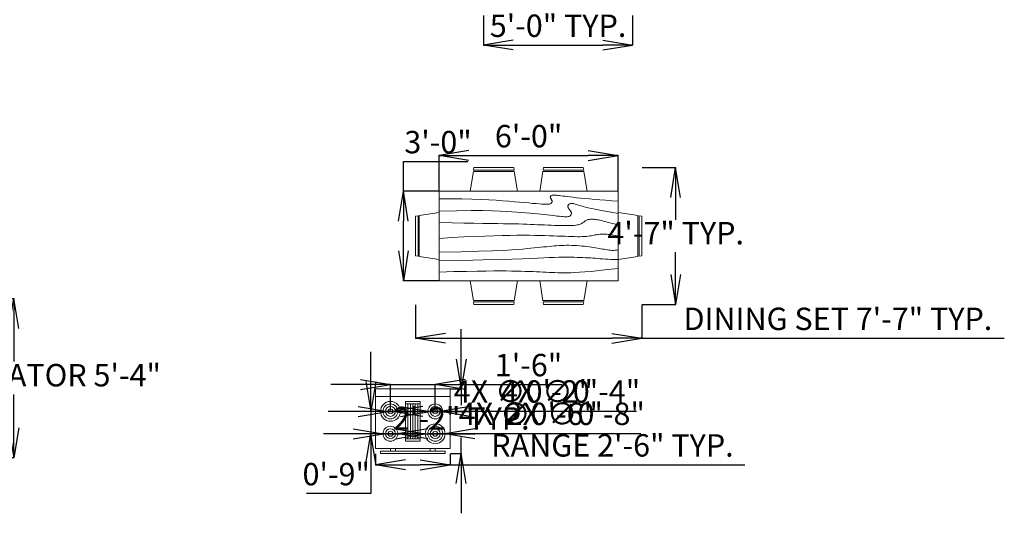
# Model space of a CAD drawing. Units: inches. Extents: x 1856 to 3350, y 1624 to 2224.
# Tile 6 of 7: x 2954 to 3350, y 1624 to 1823. Entities that reach past the tile are written whole.
import ezdxf

# ---------------------------------------------------------------- set-up
doc = ezdxf.new("R2010")
doc.units = ezdxf.units.IN
for name, color, linetype, lineweight in [('A-ANNO-DIMS', 2, 'Continuous', 18), ('A-EQPM', 3, 'Continuous', 18), ('A-FURN', 3, 'Continuous', 18)]:
    doc.layers.add(name, color=color, linetype=linetype, lineweight=lineweight)
doc.styles.get("Standard").update_dxf_attribs({"font": 'arial.ttf'})
doc.dimstyles.new('ISO-25', dxfattribs={"dimtxt": 9, "dimasz": 12, "dimexe": 0.125, "dimexo": 0.125, "dimgap": 2, "dimtad": 1, "dimtih": 1, "dimtoh": 1, "dimdec": 1, "dimzin": 11, "dimlunit": 4, "dimtxsty": 'Standard', "dimblk": 'OPEN', "dimcen": -0.125, "dimadec": 0, "dimazin": 0, "dimtfac": 1, "dimtdec": 1, "dimtmove": 0, "dimatfit": 3, "dimfxl": 1, "dimarcsym": 0})

# ---------------------------------------------------------------- blocks, each defined once
blk = doc.blocks.new('Dining Set - 36 x 72 in.')
for p, q in [((-22.2343, 26.00059), (-23.4847, 17.99762)), ((-22.2304, 26), (-5.7608, 26)), ((-22, 27.5), (-22.1562, 26.50042)), ((-5.8416, 26.5), (-22.1534, 26.5)), ((-22, 27.5), (-6, 27.5)), ((-5.8437, 26.49966), (-6, 27.5)), ((-4.5152, 17.99762), (-5.7655, 25.99926)), ((5.7657, 26.00059), (4.5153, 17.99762)), ((5.7696, 26), (22.2392, 26)), ((6, 27.5), (5.8438, 26.50042)), ((22.1584, 26.5), (5.8466, 26.5)), ((6, 27.5), (22, 27.5)), ((22.1563, 26.49966), (22, 27.5)), ((23.4848, 17.99762), (22.2345, 25.99926)), ((36, 18), (-36, 18)), ((-36, 18), (-36, -18)), ((36, -18), (36, 18)), ((-45.5, 8), (-44.5004, 8.15617)), ((-45.5, 8), (-45.5, -8)), ((-44.5, -8.15843), (-44.5, 8.15338)), ((-44.0006, 8.23428), (-35.9976, 9.48474)), ((-44, 8.23041), (-44, -8.23915)), ((44.0006, 8.23428), (35.9976, 9.48474)), ((44, 8.23041), (44, -8.23915)), ((44.5, -8.15843), (44.5, 8.15338)), ((45.5, 8), (44.5005, 8.15617)), ((45.5, 8), (45.5, -8)), ((-44.4997, -8.15631), (-45.5, -8)), ((-35.9976, -9.48476), (-43.9993, -8.2345)), ((35.9976, -9.48476), (43.9993, -8.2345)), ((44.4997, -8.15631), (45.5, -8)), ((-36, -18), (36, -18)), ((-22.2343, -26.0006), (-23.4847, -17.99762)), ((-4.5152, -17.99762), (-5.7655, -25.99928)), ((5.7657, -26.0006), (4.5153, -17.99762)), ((23.4848, -17.99762), (22.2345, -25.99928)), ((-22.2304, -26), (-5.7608, -26)), ((-22, -27.5), (-22.1562, -26.50044)), ((-5.8416, -26.5), (-22.1534, -26.5)), ((-22, -27.5), (-6, -27.5)), ((-5.8437, -26.49967), (-6, -27.5)), ((5.7696, -26), (22.2392, -26)), ((6, -27.5), (5.8438, -26.50044)), ((22.1584, -26.5), (5.8466, -26.5)), ((6, -27.5), (22, -27.5)), ((22.1563, -26.49967), (22, -27.5))]:
    blk.add_line(p, q)
for points in [[(-36, 15), (-31.1772, 14.97754), (-26.8079, 14.91406), (-22.8538, 14.81543), (-19.276, 14.6875), (-16.0362, 14.53613), (-13.0957, 14.36718), (-10.4159, 14.18652), (-7.9583, 14), (-5.6904, 13.81315), (-3.6035, 13.63021), (-1.6954, 13.45508), (0.0365, 13.29166), (1.5945, 13.14388), (2.9811, 13.01562), (4.1988, 12.9108), (5.25, 12.83333), (6.1393, 12.78613), (6.8802, 12.76823), (7.4883, 12.77767), (7.9792, 12.8125), (8.3685, 12.87077), (8.6719, 12.95052), (8.9049, 13.0498), (9.0833, 13.16666), (9.2205, 13.29899), (9.3216, 13.44401), (9.3895, 13.59879), (9.4271, 13.76041), (9.4373, 13.92594), (9.4232, 14.09245), (9.3875, 14.257), (9.3333, 14.41666), (9.2638, 14.56917), (9.1836, 14.71484), (9.0975, 14.85465), (9.0104, 14.98958), (8.9272, 15.1206), (8.8529, 15.2487), (8.7922, 15.37483), (8.75, 15.5), (8.7305, 15.62467), (8.7344, 15.74739), (8.7617, 15.86621), (8.8125, 15.97916), (8.8867, 16.08431), (8.9844, 16.17968), (9.1055, 16.26334), (9.25, 16.33333), (9.4189, 16.38802), (9.6172, 16.42708), (9.8506, 16.45052), (10.125, 16.45833), (10.4463, 16.45052), (10.8203, 16.42708), (11.2529, 16.38802), (11.75, 16.33333), (12.3184, 16.26318), (12.9694, 16.17838), (13.7151, 16.07991), (14.5677, 15.96875), (15.5395, 15.84586), (16.6426, 15.71224), (17.8893, 15.56884), (19.2917, 15.41666), (20.859, 15.25667), (22.5879, 15.08984), (24.4721, 14.91715), (26.5052, 14.73958), (28.6809, 14.5581), (30.9929, 14.3737), (33.4347, 14.18733), (36, 14)], [(-36, 10), (-28.9766, 10.14274), (-23.1725, 10.20442), (-18.4241, 10.19775), (-14.5677, 10.13541), (-11.4399, 10.03011), (-8.877, 9.89453), (-6.7154, 9.74137), (-4.7917, 9.58333), (-2.9698, 9.43082), (-1.2246, 9.28515), (0.4415, 9.14534), (2.026, 9.01041), (3.5266, 8.87939), (4.9408, 8.7513), (6.266, 8.62516), (7.5, 8.5), (8.6411, 8.37549), (9.6914, 8.2539), (10.6538, 8.13818), (11.5312, 8.03125), (12.3267, 7.93603), (13.043, 7.85547), (13.6831, 7.79248), (14.25, 7.75), (14.7471, 7.7303), (15.1797, 7.73307), (15.5537, 7.75732), (15.875, 7.80208), (16.1494, 7.86637), (16.3828, 7.94922), (16.5811, 8.04964), (16.75, 8.16666), (16.8944, 8.29915), (17.0143, 8.44531), (17.1089, 8.60319), (17.1771, 8.77083), (17.218, 8.94629), (17.2305, 9.1276), (17.2137, 9.31282), (17.1667, 9.5), (17.0895, 9.6875), (16.987, 9.875), (16.8649, 10.0625), (16.7292, 10.25), (16.5856, 10.4375), (16.4401, 10.625), (16.2985, 10.8125), (16.1667, 11), (16.05, 11.18733), (15.9518, 11.3737), (15.8752, 11.5581), (15.8229, 11.73958), (15.798, 11.91715), (15.8034, 12.08984), (15.842, 12.25667), (15.9167, 12.41666), (16.0295, 12.56836), (16.1784, 12.70833), (16.3605, 12.83268), (16.5729, 12.9375), (16.8127, 13.01888), (17.0768, 13.07291), (17.3625, 13.0957), (17.6667, 13.08333), (17.9894, 13.03312), (18.3418, 12.94726), (18.7382, 12.82918), (19.1927, 12.68229), (19.7195, 12.51001), (20.3327, 12.31575), (21.0465, 12.10294), (21.875, 11.875), (22.8357, 11.63354), (23.959, 11.37304), (25.2786, 11.08618), (26.8282, 10.76562), (28.6414, 10.40405), (30.752, 9.99414), (33.1936, 9.52856), (36, 9)], [(-36, 5.5), (-30.7157, 5.3348), (-26.069, 5.20963), (-21.9946, 5.11767), (-18.4271, 5.05208), (-15.3009, 5.00602), (-12.5508, 4.97265), (-10.1112, 4.94515), (-7.9167, 4.91666), (-5.909, 4.88167), (-4.0586, 4.83984), (-2.3429, 4.79215), (-0.7396, 4.73958), (0.7739, 4.6831), (2.22, 4.6237), (3.6213, 4.56233), (5, 4.5), (6.373, 4.43782), (7.7344, 4.3776), (9.0723, 4.32129), (10.375, 4.27083), (11.6309, 4.22819), (12.8281, 4.19531), (13.9551, 4.17415), (15, 4.16666), (15.954, 4.17448), (16.819, 4.19791), (17.6001, 4.23698), (18.3021, 4.29166), (18.9299, 4.36198), (19.4883, 4.44791), (19.9823, 4.54948), (20.4167, 4.66666), (20.7969, 4.79899), (21.1302, 4.94401), (21.4245, 5.09879), (21.6875, 5.26041), (21.9271, 5.42594), (22.1511, 5.59245), (22.3672, 5.757), (22.5834, 5.91666), (22.8065, 6.06868), (23.0404, 6.21093), (23.2879, 6.34147), (23.5521, 6.45833), (23.8358, 6.55957), (24.142, 6.64323), (24.4735, 6.70735), (24.8334, 6.75), (25.2235, 6.76969), (25.642, 6.76692), (26.0858, 6.74267), (26.5521, 6.69791), (27.0379, 6.63362), (27.5404, 6.55078), (28.0565, 6.45036), (28.5834, 6.33333), (29.1242, 6.19987), (29.7071, 6.04687), (30.3661, 5.87044), (31.1354, 5.66666), (32.0493, 5.43164), (33.142, 5.16146), (34.4475, 4.85221), (36, 4.5)], [(-36, -1), (-30.7915, -0.6591), (-26.0195, -0.38216), (-21.6519, -0.16284), (-17.6563, 0.00521), (-14.0005, 0.12833), (-10.6523, 0.21289), (-7.5796, 0.26522), (-4.75, 0.29166), (-2.134, 0.29793), (0.2878, 0.28711), (2.5317, 0.26163), (4.6146, 0.22396), (6.5529, 0.17651), (8.3633, 0.12174), (10.0623, 0.06209), (11.6667, 0), (13.1899, -0.06201), (14.6341, -0.1211), (15.9982, -0.17432), (17.2813, -0.21875), (18.4823, -0.25147), (19.6003, -0.26953), (20.6343, -0.27002), (21.5834, -0.25), (22.4481, -0.20768), (23.2357, -0.14584), (23.9549, -0.06836), (24.6146, 0.02083), (25.2235, 0.11784), (25.7904, 0.21875), (26.3241, 0.31966), (26.8334, 0.41666), (27.3265, 0.50618), (27.8099, 0.58593), (28.2894, 0.65397), (28.7709, 0.70833), (29.2601, 0.74707), (29.763, 0.76823), (30.2855, 0.76985), (30.8334, 0.75), (31.4088, 0.70784), (31.9994, 0.64713), (32.589, 0.57275), (33.1615, 0.48958), (33.7008, 0.4025), (34.1908, 0.3164), (34.6153, 0.23616), (34.9584, 0.16666), (35.2099, 0.11165), (35.3848, 0.07031), (35.504, 0.04069), (35.5886, 0.02083), (35.6594, 0.00879), (35.7377, 0.0026), (35.8442, 0.00032), (36, 0)], [(-36, -6.5), (-27.1843, -6.31267), (-20.084, -6.1263), (-14.469, -5.9419), (-10.1094, -5.76042), (-6.7752, -5.58285), (-4.2363, -5.41016), (-2.2629, -5.24333), (-0.625, -5.08334), (0.8708, -4.93099), (2.2715, -4.78646), (3.5872, -4.64974), (4.8281, -4.52084), (6.0046, -4.39974), (7.127, -4.28646), (8.2053, -4.18099), (9.25, -4.08334), (10.2705, -3.99382), (11.2734, -3.91407), (12.2647, -3.84603), (13.25, -3.79167), (14.2354, -3.75293), (15.2266, -3.73177), (16.2295, -3.73015), (17.25, -3.75), (18.2912, -3.79248), (19.3451, -3.85547), (20.4009, -3.93604), (21.4479, -4.03125), (22.4754, -4.13819), (23.4727, -4.25391), (24.4289, -4.37549), (25.3334, -4.5), (26.1785, -4.62492), (26.9694, -4.74935), (27.7145, -4.87281), (28.4219, -4.99479), (29.1, -5.11483), (29.7572, -5.23242), (30.4016, -5.34709), (31.0417, -5.45834), (31.6837, -5.56437), (32.3262, -5.65821), (32.9658, -5.73153), (33.599, -5.77604), (34.2224, -5.78345), (34.8327, -5.74545), (35.4264, -5.65373), (36, -5.5)], [(-36, -10), (-26.4022, -9.81299), (-18.4675, -9.62891), (-11.9839, -9.45069), (-6.7396, -9.28125), (-2.5226, -9.12354), (0.8789, -8.98047), (3.6769, -8.85498), (6.0833, -8.75), (8.2767, -8.66765), (10.3021, -8.60677), (12.1712, -8.56543), (13.8958, -8.54167), (15.4876, -8.53353), (16.9583, -8.53907), (18.3197, -8.55632), (19.5834, -8.58334), (20.7616, -8.61841), (21.8685, -8.66081), (22.9188, -8.71004), (23.9271, -8.76563), (24.9081, -8.82707), (25.8763, -8.89388), (26.8465, -8.96558), (27.8334, -9.04167), (28.8474, -9.12118), (29.8828, -9.20117), (30.93, -9.27824), (31.9792, -9.34896), (33.0205, -9.40991), (34.0443, -9.45768), (35.0407, -9.48885), (36, -9.5)], [(-36, -14.5), (-30.0881, -14.33513), (-25.0332, -14.21224), (-20.7312, -14.12647), (-17.0781, -14.07292), (-13.97, -14.04671), (-11.3027, -14.04297), (-8.9724, -14.05681), (-6.875, -14.08334), (-4.9224, -14.11833), (-3.0905, -14.16016), (-1.3709, -14.20785), (0.2448, -14.26042), (1.7647, -14.3169), (3.1973, -14.3763), (4.5507, -14.43767), (5.8333, -14.5), (7.0554, -14.5621), (8.235, -14.62175), (9.3922, -14.67652), (10.5469, -14.72396), (11.7192, -14.76164), (12.929, -14.78711), (14.1965, -14.79794), (15.5417, -14.79167), (16.9933, -14.76424), (18.6152, -14.70508), (20.4804, -14.60197), (22.6615, -14.44271), (25.2312, -14.21509), (28.2624, -13.9069), (31.8277, -13.50594), (36, -13)]]:
    blk.add_lwpolyline(points)
blk = doc.blocks.new('Range-Oven - 30 in top')
for p, q in [((0, -3), (30, -3)), ((12, -6), (18, -6)), ((13, -20), (13, -6)), ((14, -6), (14, -20)), ((15, -20), (15, -6)), ((16, -6), (16, -20)), ((17, -20), (17, -6)), ((18, -20), (12, -20)), ((6, -24), (6, -25)), ((8, -25), (8, -24)), ((22, -25), (22, -24)), ((24, -24), (24, -25))]:
    blk.add_line(p, q)
for points in [[(0, -24), (0, 0), (30, 0), (30, -24)], [(12, -21), (12, -5), (18, -5), (18, -21)], [(2, -26), (2, -25), (28, -25), (28, -26)]]:
    blk.add_lwpolyline(points, close=True)
for centre, radius in [((6, -9), 4), ((6, -9), 3), ((6, -9), 2), ((24, -9), 3), ((24, -9), 2), ((6, -9), 1), ((24, -9), 1), ((6, -18), 3), ((24, -18), 4), ((24, -18), 3), ((6, -18), 2), ((6, -18), 1), ((24, -18), 2), ((24, -18), 1)]:
    blk.add_circle(centre, radius)
blk = doc.blocks.new('_Open')
at = {"color": 0, "linetype": 'ByBlock', "lineweight": -2}
for p, q in [((-1, 0.167), (0, 0)), ((-1, -0.167), (0, 0)), ((0, 0), (-1, 0))]:
    blk.add_line(p, q, dxfattribs=at)
blk = doc.blocks.new('*D35')
at = {"layer": 'A-ANNO-DIMS', "color": 0, "lineweight": -2, "transparency": 16777216}
for p, q in [((3140.83, 1824.42), (3140.83, 1812.42)), ((3200.83, 1824.42), (3200.83, 1812.42)), ((3152.83, 1812.55), (3188.83, 1812.55))]:
    blk.add_line(p, q, dxfattribs=at)
at = {"layer": 'Defpoints', "color": 0, "transparency": 16777216}
for p in [(3140.83, 1824.55), (3200.83, 1824.55), (3200.83, 1812.55)]:
    blk.add_point(p, dxfattribs=at)
at = {"layer": 'A-ANNO-DIMS', "color": 0, "lineweight": -2, "transparency": 16777216, "xscale": 12, "yscale": 12, "zscale": 12, "rotation": 180}
blk.add_blockref('_Open', (3140.83, 1812.55), dxfattribs=at)
at = {"layer": 'A-ANNO-DIMS', "color": 0, "lineweight": -2, "transparency": 16777216, "xscale": 12, "yscale": 12, "zscale": 12}
blk.add_blockref('_Open', (3200.83, 1812.55), dxfattribs=at)
at = {"layer": 'A-ANNO-DIMS', "color": 0, "transparency": 16777216, "insert": (3170.83, 1819.14), "char_height": 9, "attachment_point": 5}
blk.add_mtext('5\'-0" TYP.', dxfattribs=at)
blk = doc.blocks.new('*D42')
at = {"layer": 'A-ANNO-DIMS', "color": 0, "lineweight": -2, "transparency": 16777216}
for p, q in [((3113.49, 1708.1), (3113.49, 1694.45)), ((3204.49, 1708.1), (3204.49, 1694.45)), ((3125.49, 1694.57), (3192.49, 1694.57)), ((3204.49, 1694.57), (3350.35, 1694.57))]:
    blk.add_line(p, q, dxfattribs=at)
at = {"layer": 'Defpoints', "color": 0, "transparency": 16777216}
for p in [(3113.49, 1708.22), (3204.49, 1708.22), (3204.49, 1694.57)]:
    blk.add_point(p, dxfattribs=at)
at = {"layer": 'A-ANNO-DIMS', "color": 0, "lineweight": -2, "transparency": 16777216, "xscale": 12, "yscale": 12, "zscale": 12, "rotation": 180}
blk.add_blockref('_Open', (3113.49, 1694.57), dxfattribs=at)
at = {"layer": 'A-ANNO-DIMS', "color": 0, "lineweight": -2, "transparency": 16777216, "xscale": 12, "yscale": 12, "zscale": 12}
blk.add_blockref('_Open', (3204.49, 1694.57), dxfattribs=at)
at = {"layer": 'A-ANNO-DIMS', "color": 0, "transparency": 16777216, "insert": (3283.42, 1701.23), "char_height": 9, "attachment_point": 5}
blk.add_mtext('DINING SET 7\'-7" TYP.', dxfattribs=at)
blk = doc.blocks.new('*D43')
at = {"layer": 'A-ANNO-DIMS', "color": 0, "lineweight": -2, "transparency": 16777216}
for p, q in [((3204.62, 1763.22), (3218.27, 1763.22)), ((3218.14, 1751.22), (3218.14, 1742.23)), ((3218.14, 1720.22), (3218.14, 1729.22)), ((3204.62, 1708.22), (3218.27, 1708.22))]:
    blk.add_line(p, q, dxfattribs=at)
at = {"layer": 'Defpoints', "color": 0, "transparency": 16777216}
for p in [(3204.49, 1763.22), (3218.14, 1763.22), (3204.49, 1708.22)]:
    blk.add_point(p, dxfattribs=at)
at = {"layer": 'A-ANNO-DIMS', "color": 0, "lineweight": -2, "transparency": 16777216, "xscale": 12, "yscale": 12, "zscale": 12}
for p, rotation in [((3218.14, 1763.22), 90), ((3218.14, 1708.22), 270)]:
    blk.add_blockref('_Open', p, dxfattribs=dict(at, rotation=rotation))
at = {"layer": 'A-ANNO-DIMS', "color": 0, "transparency": 16777216, "insert": (3218.14, 1735.72), "char_height": 9, "attachment_point": 5}
blk.add_mtext('4\'-7" TYP.', dxfattribs=at)
blk = doc.blocks.new('*D44')
at = {"layer": 'A-ANNO-DIMS', "color": 0, "lineweight": -2, "transparency": 16777216}
for p, q in [((3097.41, 1648.06), (3097.41, 1643.56)), ((3127.41, 1648.06), (3127.41, 1643.56)), ((3109.41, 1643.69), (3115.41, 1643.69)), ((3127.41, 1643.69), (3246.01, 1643.69))]:
    blk.add_line(p, q, dxfattribs=at)
at = {"layer": 'Defpoints', "color": 0, "transparency": 16777216}
for p in [(3097.41, 1648.19), (3127.41, 1648.19), (3127.41, 1643.69)]:
    blk.add_point(p, dxfattribs=at)
at = {"layer": 'A-ANNO-DIMS', "color": 0, "lineweight": -2, "transparency": 16777216, "xscale": 12, "yscale": 12, "zscale": 12, "rotation": 180}
blk.add_blockref('_Open', (3097.41, 1643.69), dxfattribs=at)
at = {"layer": 'A-ANNO-DIMS', "color": 0, "lineweight": -2, "transparency": 16777216, "xscale": 12, "yscale": 12, "zscale": 12}
blk.add_blockref('_Open', (3127.41, 1643.69), dxfattribs=at)
at = {"layer": 'A-ANNO-DIMS', "color": 0, "transparency": 16777216, "insert": (3192.71, 1650.34), "char_height": 9, "attachment_point": 5}
blk.add_mtext('RANGE 2\'-6" TYP.', dxfattribs=at)
blk = doc.blocks.new('*D45')
at = {"layer": 'A-ANNO-DIMS', "color": 0, "lineweight": -2, "transparency": 16777216}
for p, q in [((3131.91, 1686.19), (3131.91, 1698.19)), ((3127.53, 1674.19), (3132.03, 1674.19)), ((3131.91, 1674.19), (3131.91, 1667.71)), ((3131.91, 1648.19), (3131.91, 1654.67)), ((3127.53, 1648.19), (3132.03, 1648.19)), ((3131.91, 1636.19), (3131.91, 1624.19))]:
    blk.add_line(p, q, dxfattribs=at)
at = {"layer": 'Defpoints', "color": 0, "transparency": 16777216}
for p in [(3127.41, 1674.19), (3131.91, 1674.19), (3127.41, 1648.19)]:
    blk.add_point(p, dxfattribs=at)
at = {"layer": 'A-ANNO-DIMS', "color": 0, "lineweight": -2, "transparency": 16777216, "xscale": 12, "yscale": 12, "zscale": 12}
for p, rotation in [((3131.91, 1674.19), 270), ((3131.91, 1648.19), 90)]:
    blk.add_blockref('_Open', p, dxfattribs=dict(at, rotation=rotation))
at = {"layer": 'A-ANNO-DIMS', "color": 0, "transparency": 16777216, "insert": (3131.91, 1661.19), "char_height": 9, "attachment_point": 5}
blk.add_mtext('2\'-2" TYP.', dxfattribs=at)
blk = doc.blocks.new('*D46')
at = {"layer": 'A-ANNO-DIMS', "color": 0, "lineweight": -2, "transparency": 16777216}
for p, q in [((2942.46, 1710.58), (2952.06, 1710.58)), ((2951.94, 1698.58), (2951.94, 1685.23)), ((2951.94, 1658.58), (2951.94, 1671.92)), ((2942.46, 1646.58), (2952.06, 1646.58))]:
    blk.add_line(p, q, dxfattribs=at)
at = {"layer": 'Defpoints', "color": 0, "transparency": 16777216}
for p in [(2942.34, 1710.58), (2951.94, 1710.58), (2942.34, 1646.58)]:
    blk.add_point(p, dxfattribs=at)
at = {"layer": 'A-ANNO-DIMS', "color": 0, "lineweight": -2, "transparency": 16777216, "xscale": 12, "yscale": 12, "zscale": 12}
for p, rotation in [((2951.94, 1710.58), 90), ((2951.94, 1646.58), 270)]:
    blk.add_blockref('_Open', p, dxfattribs=dict(at, rotation=rotation))
at = {"layer": 'A-ANNO-DIMS', "color": 0, "transparency": 16777216, "insert": (2951.94, 1678.58), "char_height": 9, "attachment_point": 5}
blk.add_mtext('REFRIGERATOR 5\'-4"', dxfattribs=at)
blk = doc.blocks.new('*D77')
at = {"layer": 'A-ANNO-DIMS', "color": 0, "lineweight": -2, "transparency": 16777216}
for p, q in [((3122.99, 1753.85), (3122.99, 1768.25)), ((3134.99, 1768.12), (3182.99, 1768.12)), ((3194.99, 1753.85), (3194.99, 1768.25))]:
    blk.add_line(p, q, dxfattribs=at)
at = {"layer": 'Defpoints', "color": 0, "transparency": 16777216}
for p in [(3194.99, 1768.12), (3122.99, 1753.72), (3194.99, 1753.72)]:
    blk.add_point(p, dxfattribs=at)
at = {"layer": 'A-ANNO-DIMS', "color": 0, "lineweight": -2, "transparency": 16777216, "xscale": 12, "yscale": 12, "zscale": 12, "rotation": 180}
blk.add_blockref('_Open', (3122.99, 1768.12), dxfattribs=at)
at = {"layer": 'A-ANNO-DIMS', "color": 0, "lineweight": -2, "transparency": 16777216, "xscale": 12, "yscale": 12, "zscale": 12}
blk.add_blockref('_Open', (3194.99, 1768.12), dxfattribs=at)
at = {"layer": 'A-ANNO-DIMS', "color": 0, "transparency": 16777216, "insert": (3158.99, 1774.72), "char_height": 9, "attachment_point": 5}
blk.add_mtext('6\'-0"', dxfattribs=at)
blk = doc.blocks.new('*D78')
at = {"layer": 'A-ANNO-DIMS', "color": 0, "lineweight": -2, "transparency": 16777216}
for p, q in [((3108.59, 1753.72), (3108.59, 1765.72)), ((3108.59, 1765.72), (3134.51, 1765.72)), ((3122.87, 1753.72), (3108.47, 1753.72)), ((3108.59, 1729.72), (3108.59, 1741.72)), ((3122.87, 1717.72), (3108.47, 1717.72))]:
    blk.add_line(p, q, dxfattribs=at)
at = {"layer": 'Defpoints', "color": 0, "transparency": 16777216}
for p in [(3108.59, 1753.72), (3122.99, 1753.72), (3122.99, 1717.72)]:
    blk.add_point(p, dxfattribs=at)
at = {"layer": 'A-ANNO-DIMS', "color": 0, "lineweight": -2, "transparency": 16777216, "xscale": 12, "yscale": 12, "zscale": 12}
for p, rotation in [((3108.59, 1753.72), 90), ((3108.59, 1717.72), 270)]:
    blk.add_blockref('_Open', p, dxfattribs=dict(at, rotation=rotation))
at = {"layer": 'A-ANNO-DIMS', "color": 0, "transparency": 16777216, "insert": (3122.55, 1772.32), "char_height": 9, "attachment_point": 5}
blk.add_mtext('3\'-0"', dxfattribs=at)
blk = doc.blocks.new('*D79')
at = {"layer": 'A-ANNO-DIMS', "color": 0, "lineweight": -2, "transparency": 16777216}
for p, q in [((3091.41, 1676.04), (3079.41, 1676.04)), ((3103.41, 1665.31), (3103.41, 1676.16)), ((3103.41, 1676.04), (3121.41, 1676.04)), ((3121.41, 1665.31), (3121.41, 1676.16)), ((3133.41, 1676.04), (3172.49, 1676.04))]:
    blk.add_line(p, q, dxfattribs=at)
at = {"layer": 'Defpoints', "color": 0, "transparency": 16777216}
for p in [(3121.41, 1676.04), (3103.41, 1665.19), (3121.41, 1665.19)]:
    blk.add_point(p, dxfattribs=at)
at = {"layer": 'A-ANNO-DIMS', "color": 0, "lineweight": -2, "transparency": 16777216, "xscale": 12, "yscale": 12, "zscale": 12}
blk.add_blockref('_Open', (3103.41, 1676.04), dxfattribs=at)
at = {"layer": 'A-ANNO-DIMS', "color": 0, "lineweight": -2, "transparency": 16777216, "xscale": 12, "yscale": 12, "zscale": 12, "rotation": 180}
blk.add_blockref('_Open', (3121.41, 1676.04), dxfattribs=at)
at = {"layer": 'A-ANNO-DIMS', "color": 0, "transparency": 16777216, "insert": (3158.95, 1682.63), "char_height": 9, "attachment_point": 5}
blk.add_mtext('1\'-6"', dxfattribs=at)
blk = doc.blocks.new('*D80')
at = {"layer": 'A-ANNO-DIMS', "color": 0, "lineweight": -2, "transparency": 16777216}
for p, q in [((3095.56, 1677.19), (3095.56, 1689.19)), ((3103.28, 1665.19), (3095.43, 1665.19)), ((3095.56, 1665.19), (3095.56, 1656.19)), ((3103.28, 1656.19), (3095.43, 1656.19)), ((3095.56, 1644.19), (3095.56, 1632.19)), ((3095.56, 1632.19), (3069.63, 1632.19))]:
    blk.add_line(p, q, dxfattribs=at)
at = {"layer": 'Defpoints', "color": 0, "transparency": 16777216}
for p in [(3103.41, 1665.19), (3095.56, 1656.19), (3103.41, 1656.19)]:
    blk.add_point(p, dxfattribs=at)
at = {"layer": 'A-ANNO-DIMS', "color": 0, "lineweight": -2, "transparency": 16777216, "xscale": 12, "yscale": 12, "zscale": 12}
for p, rotation in [((3095.56, 1665.19), 270), ((3095.56, 1656.19), 90)]:
    blk.add_blockref('_Open', p, dxfattribs=dict(at, rotation=rotation))
at = {"layer": 'A-ANNO-DIMS', "color": 0, "transparency": 16777216, "insert": (3081.6, 1638.78), "char_height": 9, "attachment_point": 5}
blk.add_mtext('0\'-9"', dxfattribs=at)
blk = doc.blocks.new('*D97')
at = {"layer": 'A-ANNO-DIMS', "color": 0, "lineweight": -2, "transparency": 16777216}
for p, q in [((3105.41, 1656.19), (3093.41, 1656.19)), ((3117.41, 1656.19), (3125.41, 1656.19)), ((3149.41, 1656.19), (3137.41, 1656.19)), ((3204.14, 1656.19), (3149.41, 1656.19))]:
    blk.add_line(p, q, dxfattribs=at)
at = {"layer": 'Defpoints', "color": 0, "transparency": 16777216}
for p in [(3117.41, 1656.19), (3125.41, 1656.19)]:
    blk.add_point(p, dxfattribs=at)
at = {"layer": 'A-ANNO-DIMS', "color": 0, "lineweight": -2, "transparency": 16777216, "xscale": 12, "yscale": 12, "zscale": 12}
for p, rotation in [((3117.41, 1656.19), 0.0034234228213048), ((3125.41, 1656.19), 180.0034234228213)]:
    blk.add_blockref('_Open', p, dxfattribs=dict(at, rotation=rotation))
at = {"layer": 'A-ANNO-DIMS', "color": 0, "transparency": 16777216, "insert": (3177.77, 1663.04), "char_height": 9, "attachment_point": 5}
blk.add_mtext('2X ∅0\'-8"', dxfattribs=at)
blk = doc.blocks.new('*D98')
at = {"layer": 'A-ANNO-DIMS', "color": 0, "lineweight": -2, "transparency": 16777216}
for p, q in [((3088.41, 1656.19), (3076.41, 1656.19)), ((3100.41, 1656.19), (3106.41, 1656.19)), ((3130.41, 1656.19), (3118.41, 1656.19)), ((3185.35, 1656.19), (3130.41, 1656.19))]:
    blk.add_line(p, q, dxfattribs=at)
at = {"layer": 'Defpoints', "color": 0, "transparency": 16777216}
for p in [(3100.41, 1656.19), (3106.41, 1656.19)]:
    blk.add_point(p, dxfattribs=at)
at = {"layer": 'A-ANNO-DIMS', "color": 0, "lineweight": -2, "transparency": 16777216, "xscale": 12, "yscale": 12, "zscale": 12}
for p, rotation in [((3100.41, 1656.19), 0.0045645637553715), ((3106.41, 1656.19), 180.0045645637553)]:
    blk.add_blockref('_Open', p, dxfattribs=dict(at, rotation=rotation))
at = {"layer": 'A-ANNO-DIMS', "color": 0, "transparency": 16777216, "insert": (3158.88, 1663.04), "char_height": 9, "attachment_point": 5}
blk.add_mtext('4X ∅0\'-6"', dxfattribs=at)
blk = doc.blocks.new('*D99')
at = {"layer": 'A-ANNO-DIMS', "color": 0, "lineweight": -2, "transparency": 16777216}
for p, q in [((3107.41, 1665.19), (3095.41, 1665.19)), ((3119.41, 1665.19), (3123.41, 1665.19)), ((3147.41, 1665.19), (3135.41, 1665.19)), ((3202.35, 1665.19), (3147.41, 1665.19))]:
    blk.add_line(p, q, dxfattribs=at)
at = {"layer": 'Defpoints', "color": 0, "transparency": 16777216}
for p in [(3119.41, 1665.19), (3123.41, 1665.19)]:
    blk.add_point(p, dxfattribs=at)
at = {"layer": 'A-ANNO-DIMS', "color": 0, "lineweight": -2, "transparency": 16777216, "xscale": 12, "yscale": 12, "zscale": 12}
for p, rotation in [((3119.41, 1665.19), 0.0068468456182291), ((3123.41, 1665.19), 180.0068468456182)]:
    blk.add_blockref('_Open', p, dxfattribs=dict(at, rotation=rotation))
at = {"layer": 'A-ANNO-DIMS', "color": 0, "transparency": 16777216, "insert": (3175.88, 1672.04), "char_height": 9, "attachment_point": 5}
blk.add_mtext('4X ∅0\'-4"', dxfattribs=at)
blk = doc.blocks.new('*D100')
at = {"layer": 'A-ANNO-DIMS', "color": 0, "lineweight": -2, "transparency": 16777216}
for p, q in [((3090.41, 1665.19), (3078.41, 1665.18)), ((3102.41, 1665.19), (3104.41, 1665.19)), ((3128.41, 1665.19), (3116.41, 1665.19)), ((3183.35, 1665.19), (3128.41, 1665.19))]:
    blk.add_line(p, q, dxfattribs=at)
at = {"layer": 'Defpoints', "color": 0, "transparency": 16777216}
for p in [(3102.41, 1665.19), (3104.41, 1665.19)]:
    blk.add_point(p, dxfattribs=at)
at = {"layer": 'A-ANNO-DIMS', "color": 0, "lineweight": -2, "transparency": 16777216, "xscale": 12, "yscale": 12, "zscale": 12}
for p, rotation in [((3102.41, 1665.19), 0.0136936910408547), ((3104.41, 1665.19), 180.0136936910408)]:
    blk.add_blockref('_Open', p, dxfattribs=dict(at, rotation=rotation))
at = {"layer": 'A-ANNO-DIMS', "color": 0, "transparency": 16777216, "insert": (3156.88, 1672.04), "char_height": 9, "attachment_point": 5}
blk.add_mtext('4X ∅0\'-2"', dxfattribs=at)

msp = doc.modelspace()

# ---------------------------------------------------------------- block references
at = {"layer": 'A-EQPM'}
msp.add_blockref('Range-Oven - 30 in top', (3097.41, 1674.19), dxfattribs=at)
at = {"layer": 'A-FURN'}
msp.add_blockref('Dining Set - 36 x 72 in.', (3158.99, 1735.72), dxfattribs=at)

# ---------------------------------------------------------------- dimensions: what is measured, and where the dimension line sits
at = {"layer": 'A-ANNO-DIMS'}
for base, p1, p2, text, picture, middle in [((3200.83, 1812.55), (3140.83, 1824.55), (3200.83, 1824.55), '<> TYP.', '*D35', (3170.83, 1819.14)), ((3204.49, 1694.57), (3113.49, 1708.22), (3204.49, 1708.22), 'DINING SET <> TYP.', '*D42', (3283.42, 1701.23)), ((3127.41, 1643.69), (3097.41, 1648.19), (3127.41, 1648.19), 'RANGE <> TYP.', '*D44', (3192.71, 1650.34))]:
    dim = msp.add_linear_dim(base=base, p1=p1, p2=p2, text=text, dimstyle='ISO-25', override={"dimdec": 1, "dimlfac": 1, "dimrnd": 0, "dimzin": 1, "dimdsep": 46, "dimlunit": 4, "dimfrac": 2}, dxfattribs=at)
    dim.commit()
    dim.dimension.update_dxf_attribs({"geometry": picture, "text_midpoint": middle})
for base, p1, p2, picture, middle in [((3194.99, 1768.12), (3122.99, 1753.72), (3194.99, 1753.72), '*D77', (3158.99, 1774.72)), ((3121.41, 1676.04), (3103.41, 1665.19), (3121.41, 1665.19), '*D79', (3158.95, 1682.63))]:
    dim = msp.add_linear_dim(base=base, p1=p1, p2=p2, dimstyle='ISO-25', override={"dimdec": 1, "dimlfac": 1, "dimrnd": 0, "dimzin": 1, "dimdsep": 46, "dimlunit": 4, "dimfrac": 2}, dxfattribs=at)
    dim.commit()
    dim.dimension.update_dxf_attribs({"geometry": picture, "text_midpoint": middle})
for base, p1, p2, picture, middle in [((3108.59, 1753.72), (3122.99, 1717.72), (3122.99, 1753.72), '*D78', (3122.55, 1772.32)), ((3095.56, 1656.19), (3103.41, 1665.19), (3103.41, 1656.19), '*D80', (3081.6, 1638.78))]:
    dim = msp.add_linear_dim(base=base, p1=p1, p2=p2, angle=90, dimstyle='ISO-25', override={"dimdec": 1, "dimlfac": 1, "dimrnd": 0, "dimzin": 1, "dimdsep": 46, "dimlunit": 4, "dimfrac": 2}, dxfattribs=at)
    dim.commit()
    dim.dimension.update_dxf_attribs({"geometry": picture, "text_midpoint": middle})
for base, p1, p2, text, picture, middle in [((3218.14, 1763.22), (3204.49, 1708.22), (3204.49, 1763.22), '<> TYP.', '*D43', (3218.14, 1735.72)), ((2951.94, 1710.58), (2942.34, 1646.58), (2942.34, 1710.58), 'REFRIGERATOR <>', '*D46', (2951.94, 1678.58)), ((3131.91, 1674.19), (3127.41, 1648.19), (3127.41, 1674.19), '<> TYP.', '*D45', (3131.91, 1661.19))]:
    dim = msp.add_linear_dim(base=base, p1=p1, p2=p2, angle=90, text=text, dimstyle='ISO-25', override={"dimdec": 1, "dimlfac": 1, "dimrnd": 0, "dimzin": 1, "dimdsep": 46, "dimlunit": 4, "dimfrac": 2}, dxfattribs=at)
    dim.commit()
    dim.dimension.update_dxf_attribs({"geometry": picture, "text_midpoint": middle})
dim = msp.add_diameter_dim_2p(p1=(3102.41, 1665.19), p2=(3104.41, 1665.19), text='4X <>', dimstyle='ISO-25', override={"dimdec": 1, "dimlfac": 1, "dimrnd": 0, "dimzin": 1, "dimdsep": 46, "dimlunit": 4, "dimfrac": 2}, dxfattribs=at)
dim.commit()
dim.dimension.update_dxf_attribs({"geometry": '*D100', "text_midpoint": (3128.41, 1665.19)})
for p1, p2, text, picture, middle in [((3119.41, 1665.19), (3123.41, 1665.19), '4X <>', '*D99', (3147.41, 1665.19)), ((3100.41, 1656.19), (3106.41, 1656.19), '4X <>', '*D98', (3130.41, 1656.19)), ((3117.41, 1656.19), (3125.41, 1656.19), '2X <>', '*D97', (3149.41, 1656.19))]:
    dim = msp.add_diameter_dim_2p(p1=p1, p2=p2, text=text, dimstyle='ISO-25', override={"dimdec": 1, "dimlfac": 1, "dimrnd": 0, "dimzin": 1, "dimdsep": 46, "dimlunit": 4, "dimfrac": 2}, dxfattribs=at)
    dim.commit()
    dim.dimension.update_dxf_attribs({"geometry": picture, "text_midpoint": middle, "dimtype": 163})

doc.saveas('drawing.dxf')
